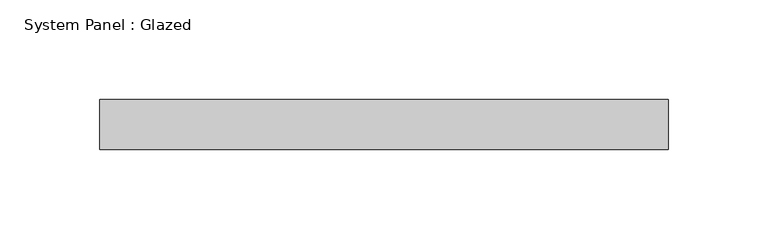
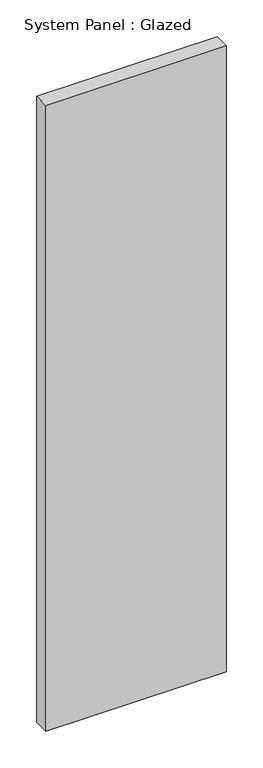
"""IFC4 building model written with IfcOpenShell, lengths in millimetres: plate geometry, System Panel : Glazed."""

from ifc_helpers import new_model, si_unit, origin, origin_with_axes, place, context, project, spatial, polyline, outline, extrude, source, transform, mapped, element, save


def system_panel_glazed_6933bc29(model_context):
    return source(origin(), model_context, "Body", "SweptSolid", [
        extrude(outline(polyline([(142.0172969, 24.5), (-142.0172969, 24.5), (-142.0172969, 49.5), (142.0172969, 49.5), (142.0172969, 24.5)])), origin_with_axes(), (0.0, 0.0, 1.0), 1041.4),
    ])


if __name__ == "__main__":
    model = new_model("IFC4")
    model_context = context("Model", 3, world=origin())
    ifc_project = project(units=[si_unit("LENGTHUNIT", "METRE", prefix="MILLI")], contexts=[model_context])
    site = spatial("IfcSite", under=ifc_project)
    building = spatial("IfcBuilding", under=site)
    placement = place(None, origin())
    system_panel_glazed_shape = system_panel_glazed_6933bc29(model_context)
    element("IfcPlate", 1, ObjectType="System Panel : Glazed", at=placement, inside=building, context=model_context, shape_type="MappedRepresentation", body=[
        mapped(system_panel_glazed_shape, transform((0.0, 0.0, 0.0), x_axis=(1.0, 0.0, 0.0), y_axis=(0.0, 1.0, 0.0), z_axis=(0.0, 0.0, 1.0))),
    ])
    save(model, "model.ifc")

# Revit data of these elements
# Type "System Panel : Glazed"
#   Keynote = "H11"
#   Construction Type Id = "GSP4R"
#   Analytic Construction = "1/8 in Pilkington single glazing"
#   Visual Light Transmittance = 0.9
#   Solar Heat Gain Coefficient = 0.86
#   Heat Transfer Coefficient (U) = 6.7069 W/(m²·K)
#   Define Thermal Properties by = 1
# Element 1 (IfcPlate, "System Panel : Glazed")
#   Materials on its faces: "Glass"
# Materials
#   "Glass": class "Glass", colour RGB 0 128 192, transparency 0.9, Description = "Soda Lime Glass", Cost = 0
